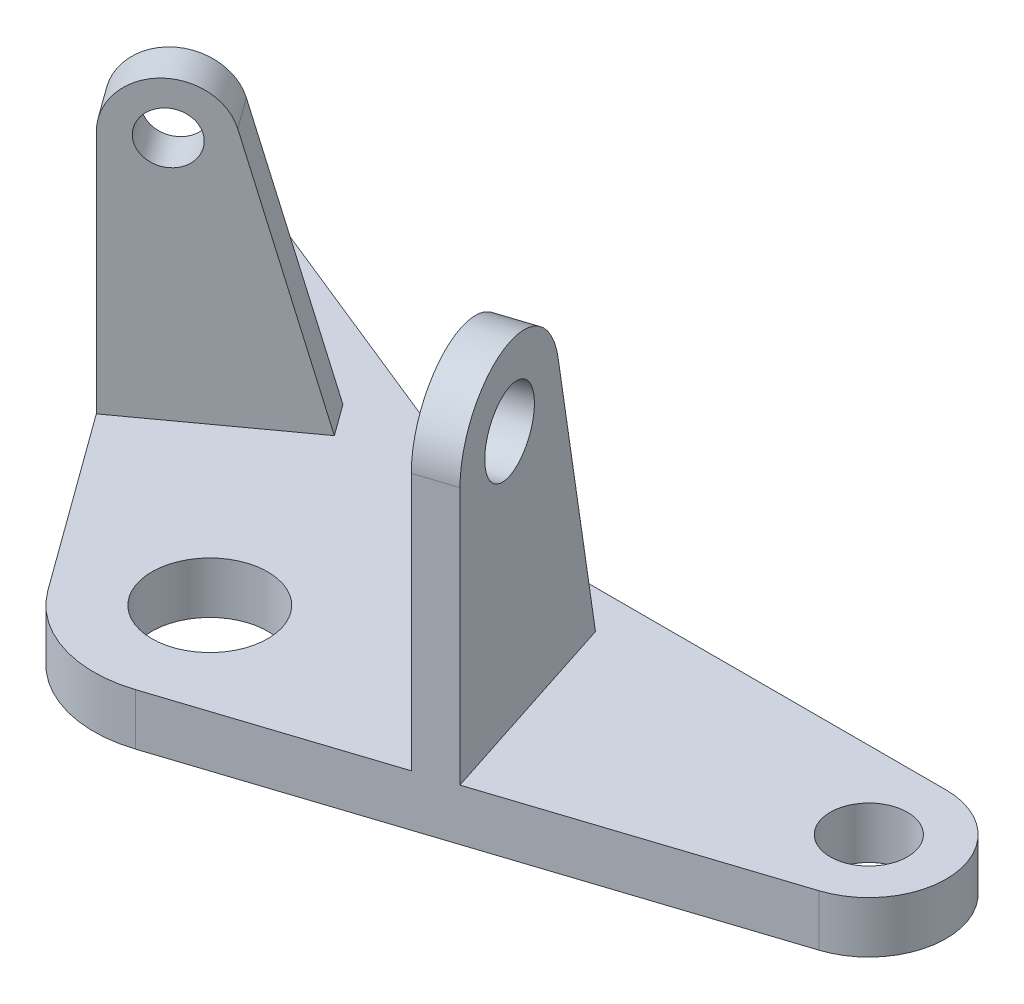
ISO-10303-21;
HEADER;
FILE_DESCRIPTION(('STEP AP214'),'2;1');
FILE_NAME('part.step','',(''),(''),'','','');
FILE_SCHEMA(('AUTOMOTIVE_DESIGN { 1 0 10303 214 1 1 1 1 }'));
ENDSEC;
DATA;
#1=APPLICATION_CONTEXT('core data for automotive mechanical design processes');
#2=APPLICATION_PROTOCOL_DEFINITION('international standard','automotive_design',2000,#1);
#3=PRODUCT_CONTEXT('',#1,'mechanical');
#4=PRODUCT('Part','Part','',(#3));
#5=PRODUCT_RELATED_PRODUCT_CATEGORY('part','',(#4));
#6=PRODUCT_DEFINITION_FORMATION('','',#4);
#7=PRODUCT_DEFINITION_CONTEXT('part definition',#1,'design');
#8=PRODUCT_DEFINITION('design','',#6,#7);
#9=PRODUCT_DEFINITION_SHAPE('','',#8);
#10=(LENGTH_UNIT() NAMED_UNIT(*) SI_UNIT(.MILLI.,.METRE.));
#11=(NAMED_UNIT(*) PLANE_ANGLE_UNIT() SI_UNIT($,.RADIAN.));
#12=(NAMED_UNIT(*) SI_UNIT($,.STERADIAN.) SOLID_ANGLE_UNIT());
#13=UNCERTAINTY_MEASURE_WITH_UNIT(LENGTH_MEASURE(1.E-05),#10,'distance_accuracy_value','');
#14=(GEOMETRIC_REPRESENTATION_CONTEXT(3) GLOBAL_UNCERTAINTY_ASSIGNED_CONTEXT((#13)) GLOBAL_UNIT_ASSIGNED_CONTEXT((#10,
#11,#12)) REPRESENTATION_CONTEXT('',''));
#15=CARTESIAN_POINT('',(0.,0.,0.));
#16=DIRECTION('',(0.,0.,1.));
#17=DIRECTION('',(1.,0.,0.));
#18=AXIS2_PLACEMENT_3D('',#15,#16,#17);
#19=CARTESIAN_POINT('',(82.,8.,-20.3346417456688));
#20=DIRECTION('',(0.,1.,0.));
#21=DIRECTION('',(0.,0.,1.));
#22=AXIS2_PLACEMENT_3D('',#19,#20,#21);
#23=PLANE('',#22);
#24=CARTESIAN_POINT('',(0.,8.,0.));
#25=DIRECTION('',(0.,1.,0.));
#26=DIRECTION('',(0.,0.,1.));
#27=AXIS2_PLACEMENT_3D('',#24,#25,#26);
#28=CIRCLE('',#27,9.);
#29=CARTESIAN_POINT('',(0.,8.,9.));
#30=VERTEX_POINT('',#29);
#31=EDGE_CURVE('E231',#30,#30,#28,.T.);
#32=ORIENTED_EDGE('',*,*,#31,.F.);
#33=EDGE_LOOP('',(#32));
#34=FACE_BOUND('',#33,.T.);
#35=CARTESIAN_POINT('',(82.,8.,-20.3346417456688));
#36=DIRECTION('',(0.,1.,0.));
#37=DIRECTION('',(0.,0.,1.));
#38=AXIS2_PLACEMENT_3D('',#35,#36,#37);
#39=CIRCLE('',#38,6.);
#40=CARTESIAN_POINT('',(82.,8.,-14.3346417456688));
#41=VERTEX_POINT('',#40);
#42=EDGE_CURVE('E227',#41,#41,#39,.T.);
#43=ORIENTED_EDGE('',*,*,#42,.F.);
#44=EDGE_LOOP('',(#43));
#45=FACE_BOUND('',#44,.T.);
#46=CARTESIAN_POINT('',(-48.,8.,-49.0533160155749));
#47=DIRECTION('',(0.,1.,0.));
#48=DIRECTION('',(0.,0.,1.));
#49=AXIS2_PLACEMENT_3D('',#46,#47,#48);
#50=CIRCLE('',#49,4.00000000000001);
#51=CARTESIAN_POINT('',(-48.,8.,-45.0533160155749));
#52=VERTEX_POINT('',#51);
#53=EDGE_CURVE('E223',#52,#52,#50,.T.);
#54=ORIENTED_EDGE('',*,*,#53,.F.);
#55=EDGE_LOOP('',(#54));
#56=FACE_BOUND('',#55,.T.);
#57=DIRECTION('',(0.309016994374949,0.,0.951056516295153));
#58=VECTOR('',#57,1.);
#59=CARTESIAN_POINT('',(37.8982274527843,8.,6.6124394845645));
#60=LINE('',#59,#58);
#61=CARTESIAN_POINT('',(27.7716325131749,8.,-24.5540150487136));
#62=VERTEX_POINT('',#61);
#63=CARTESIAN_POINT('',(37.8982274527843,8.,6.6124394845645));
#64=VERTEX_POINT('',#63);
#65=EDGE_CURVE('E54',#62,#64,#60,.T.);
#66=ORIENTED_EDGE('',*,*,#65,.F.);
#67=DIRECTION('',(0.951056516295153,0.,-0.309016994374949));
#68=VECTOR('',#67,1.);
#69=CARTESIAN_POINT('',(27.7716325131749,8.,-24.5540150487136));
#70=LINE('',#69,#68);
#71=CARTESIAN_POINT('',(33.4779716109458,8.,-26.4081170149633));
#72=VERTEX_POINT('',#71);
#73=EDGE_CURVE('E180',#62,#72,#70,.T.);
#74=ORIENTED_EDGE('',*,*,#73,.T.);
#75=DIRECTION('',(-0.309016994374949,0.,-0.951056516295153));
#76=VECTOR('',#75,1.);
#77=CARTESIAN_POINT('',(34.1624443371439,8.,-24.3015265738979));
#78=LINE('',#77,#76);
#79=CARTESIAN_POINT('',(43.6045665505552,8.,4.75833751831482));
#80=VERTEX_POINT('',#79);
#81=EDGE_CURVE('E64',#80,#72,#78,.T.);
#82=ORIENTED_EDGE('',*,*,#81,.F.);
#83=DIRECTION('',(0.951056516295153,0.,-0.309016994374949));
#84=VECTOR('',#83,1.);
#85=CARTESIAN_POINT('',(85.7082039324994,8.,-8.92196355012698));
#86=LINE('',#85,#84);
#87=CARTESIAN_POINT('',(85.7082039324994,8.,-8.92196355012698));
#88=VERTEX_POINT('',#87);
#89=EDGE_CURVE('E260',#80,#88,#86,.T.);
#90=ORIENTED_EDGE('',*,*,#89,.T.);
#91=CARTESIAN_POINT('',(82.,8.,-20.3346417456688));
#92=DIRECTION('',(0.,1.,0.));
#93=DIRECTION('',(0.,0.,1.));
#94=AXIS2_PLACEMENT_3D('',#91,#92,#93);
#95=CIRCLE('',#94,12.);
#96=CARTESIAN_POINT('',(82.,8.,-32.3346417456688));
#97=VERTEX_POINT('',#96);
#98=EDGE_CURVE('E237',#88,#97,#95,.T.);
#99=ORIENTED_EDGE('',*,*,#98,.T.);
#100=DIRECTION('',(-1.,0.,0.));
#101=VECTOR('',#100,1.);
#102=CARTESIAN_POINT('',(82.,8.,-32.3346417456688));
#103=LINE('',#102,#101);
#104=CARTESIAN_POINT('',(22.8998811762112,8.,-32.3346417456688));
#105=VERTEX_POINT('',#104);
#106=EDGE_CURVE('E245',#97,#105,#103,.T.);
#107=ORIENTED_EDGE('',*,*,#106,.T.);
#108=CARTESIAN_POINT('',(22.899881176211,8.,-74.3346417456688));
#109=DIRECTION('',(0.,-1.,0.));
#110=DIRECTION('',(0.,0.,-1.));
#111=AXIS2_PLACEMENT_3D('',#108,#109,#110);
#112=CIRCLE('',#111,42.);
#113=CARTESIAN_POINT('',(7.16640425274284,8.,-35.3929198538637));
#114=VERTEX_POINT('',#113);
#115=EDGE_CURVE('E244',#105,#114,#112,.T.);
#116=ORIENTED_EDGE('',*,*,#115,.T.);
#117=DIRECTION('',(-0.92718385456679,0.,-0.374606593415906));
#118=VECTOR('',#117,1.);
#119=CARTESIAN_POINT('',(-45.0031472526728,8.,-56.4707868521092));
#120=LINE('',#119,#118);
#121=CARTESIAN_POINT('',(-45.0031472526728,8.,-56.4707868521092));
#122=VERTEX_POINT('',#121);
#123=EDGE_CURVE('E250',#114,#122,#120,.T.);
#124=ORIENTED_EDGE('',*,*,#123,.T.);
#125=CARTESIAN_POINT('',(-48.,8.,-49.0533160155749));
#126=DIRECTION('',(0.,1.,0.));
#127=DIRECTION('',(0.,0.,1.));
#128=AXIS2_PLACEMENT_3D('',#125,#126,#127);
#129=CIRCLE('',#128,8.);
#130=CARTESIAN_POINT('',(-54.4721359549996,8.,-44.3510339972351));
#131=VERTEX_POINT('',#130);
#132=EDGE_CURVE('E248',#122,#131,#129,.T.);
#133=ORIENTED_EDGE('',*,*,#132,.T.);
#134=DIRECTION('',(0.587785252292478,0.,0.809016994374944));
#135=VECTOR('',#134,1.);
#136=CARTESIAN_POINT('',(-54.4721359549996,8.,-44.3510339972351));
#137=LINE('',#136,#135);
#138=CARTESIAN_POINT('',(-38.0737159904481,8.,-21.7805452337331));
#139=VERTEX_POINT('',#138);
#140=EDGE_CURVE('E255',#131,#139,#137,.T.);
#141=ORIENTED_EDGE('',*,*,#140,.T.);
#142=DIRECTION('',(-0.809016994374942,0.,0.58778525229248));
#143=VECTOR('',#142,1.);
#144=CARTESIAN_POINT('',(-14.333683815428,8.,-39.0286882251011));
#145=LINE('',#144,#143);
#146=CARTESIAN_POINT('',(-16.6636647332408,8.,-37.3358579988691));
#147=VERTEX_POINT('',#146);
#148=EDGE_CURVE('E206',#147,#139,#145,.T.);
#149=ORIENTED_EDGE('',*,*,#148,.F.);
#150=DIRECTION('',(-0.58778525229248,0.,-0.809016994374942));
#151=VECTOR('',#150,1.);
#152=CARTESIAN_POINT('',(40.9392899914223,8.,41.9478074498752));
#153=LINE('',#152,#151);
#154=CARTESIAN_POINT('',(-13.1369532194859,8.,-32.4817560326195));
#155=VERTEX_POINT('',#154);
#156=EDGE_CURVE('E189',#155,#147,#153,.T.);
#157=ORIENTED_EDGE('',*,*,#156,.F.);
#158=DIRECTION('',(0.809016994374942,0.,-0.58778525229248));
#159=VECTOR('',#158,1.);
#160=CARTESIAN_POINT('',(-34.5470044766932,8.,-16.9264432674835));
#161=LINE('',#160,#159);
#162=CARTESIAN_POINT('',(-34.5470044766932,8.,-16.9264432674835));
#163=VERTEX_POINT('',#162);
#164=EDGE_CURVE('E202',#163,#155,#161,.T.);
#165=ORIENTED_EDGE('',*,*,#164,.F.);
#166=CARTESIAN_POINT('',(-14.562305898749,8.,10.5801345412646));
#167=VERTEX_POINT('',#166);
#168=EDGE_CURVE('E252',#163,#167,#137,.T.);
#169=ORIENTED_EDGE('',*,*,#168,.T.);
#170=CARTESIAN_POINT('',(0.,8.,0.));
#171=DIRECTION('',(0.,1.,0.));
#172=DIRECTION('',(0.,0.,1.));
#173=AXIS2_PLACEMENT_3D('',#170,#171,#172);
#174=CIRCLE('',#173,18.);
#175=CARTESIAN_POINT('',(5.56230589874908,8.,17.1190172933128));
#176=VERTEX_POINT('',#175);
#177=EDGE_CURVE('E253',#167,#176,#174,.T.);
#178=ORIENTED_EDGE('',*,*,#177,.T.);
#179=EDGE_CURVE('E259',#176,#64,#86,.T.);
#180=ORIENTED_EDGE('',*,*,#179,.T.);
#181=EDGE_LOOP('',(#66,#74,#82,#90,#99,#107,#116,#124,#133,#141,#149,#157,#165,#169,#178,#180));
#182=FACE_BOUND('',#181,.T.);
#183=ADVANCED_FACE('F39',(#34,#45,#56,#182),#23,.T.);
#184=CARTESIAN_POINT('',(-54.4721359549996,8.,-44.3510339972351));
#185=DIRECTION('',(0.809016994374944,0.,-0.587785252292478));
#186=DIRECTION('',(-0.587785252292478,0.,-0.809016994374944));
#187=AXIS2_PLACEMENT_3D('',#184,#185,#186);
#188=PLANE('',#187);
#189=DIRECTION('',(-0.58778525229248,0.,-0.809016994374942));
#190=VECTOR('',#189,1.);
#191=CARTESIAN_POINT('',(19.529238734215,46.,57.5031202150112));
#192=LINE('',#191,#190);
#193=CARTESIAN_POINT('',(-34.5470044766932,46.,-16.9264432674835));
#194=VERTEX_POINT('',#193);
#195=CARTESIAN_POINT('',(-38.0737159904481,46.,-21.7805452337331));
#196=VERTEX_POINT('',#195);
#197=EDGE_CURVE('E186',#194,#196,#192,.T.);
#198=ORIENTED_EDGE('',*,*,#197,.T.);
#199=DIRECTION('',(0.,-1.,0.));
#200=VECTOR('',#199,1.);
#201=CARTESIAN_POINT('',(-38.0737159904481,106.,-21.7805452337331));
#202=LINE('',#201,#200);
#203=EDGE_CURVE('E212',#196,#139,#202,.T.);
#204=ORIENTED_EDGE('',*,*,#203,.T.);
#205=ORIENTED_EDGE('',*,*,#140,.F.);
#206=DIRECTION('',(0.,-1.,0.));
#207=VECTOR('',#206,1.);
#208=CARTESIAN_POINT('',(-54.4721359549996,8.,-44.3510339972351));
#209=LINE('',#208,#207);
#210=CARTESIAN_POINT('',(-54.4721359549996,0.,-44.3510339972351));
#211=VERTEX_POINT('',#210);
#212=EDGE_CURVE('E283',#131,#211,#209,.T.);
#213=ORIENTED_EDGE('',*,*,#212,.T.);
#214=DIRECTION('',(0.587785252292478,0.,0.809016994374944));
#215=VECTOR('',#214,1.);
#216=CARTESIAN_POINT('',(-54.4721359549996,0.,-44.3510339972351));
#217=LINE('',#216,#215);
#218=CARTESIAN_POINT('',(-14.562305898749,0.,10.5801345412646));
#219=VERTEX_POINT('',#218);
#220=EDGE_CURVE('E272',#211,#219,#217,.T.);
#221=ORIENTED_EDGE('',*,*,#220,.T.);
#222=DIRECTION('',(0.,-1.,0.));
#223=VECTOR('',#222,1.);
#224=CARTESIAN_POINT('',(-14.562305898749,8.,10.5801345412646));
#225=LINE('',#224,#223);
#226=EDGE_CURVE('E284',#167,#219,#225,.T.);
#227=ORIENTED_EDGE('',*,*,#226,.F.);
#228=ORIENTED_EDGE('',*,*,#168,.F.);
#229=DIRECTION('',(0.,-1.,0.));
#230=VECTOR('',#229,1.);
#231=CARTESIAN_POINT('',(-34.5470044766932,106.,-16.9264432674835));
#232=LINE('',#231,#230);
#233=EDGE_CURVE('E214',#194,#163,#232,.T.);
#234=ORIENTED_EDGE('',*,*,#233,.F.);
#235=EDGE_LOOP('',(#198,#204,#205,#213,#221,#227,#228,#234));
#236=FACE_BOUND('',#235,.T.);
#237=ADVANCED_FACE('F334',(#236),#188,.F.);
#238=CARTESIAN_POINT('',(82.,0.,-20.3346417456688));
#239=DIRECTION('',(0.,1.,0.));
#240=DIRECTION('',(0.,0.,1.));
#241=AXIS2_PLACEMENT_3D('',#238,#239,#240);
#242=PLANE('',#241);
#243=CARTESIAN_POINT('',(82.,0.,-20.3346417456688));
#244=DIRECTION('',(0.,1.,0.));
#245=DIRECTION('',(0.,0.,1.));
#246=AXIS2_PLACEMENT_3D('',#243,#244,#245);
#247=CIRCLE('',#246,12.);
#248=CARTESIAN_POINT('',(85.7082039324994,0.,-8.92196355012698));
#249=VERTEX_POINT('',#248);
#250=CARTESIAN_POINT('',(82.,0.,-32.3346417456688));
#251=VERTEX_POINT('',#250);
#252=EDGE_CURVE('E236',#249,#251,#247,.T.);
#253=ORIENTED_EDGE('',*,*,#252,.F.);
#254=DIRECTION('',(0.951056516295153,0.,-0.309016994374949));
#255=VECTOR('',#254,1.);
#256=CARTESIAN_POINT('',(85.7082039324994,0.,-8.92196355012698));
#257=LINE('',#256,#255);
#258=CARTESIAN_POINT('',(5.56230589874908,0.,17.1190172933128));
#259=VERTEX_POINT('',#258);
#260=EDGE_CURVE('E243',#259,#249,#257,.T.);
#261=ORIENTED_EDGE('',*,*,#260,.F.);
#262=CARTESIAN_POINT('',(0.,0.,0.));
#263=DIRECTION('',(0.,1.,0.));
#264=DIRECTION('',(0.,0.,1.));
#265=AXIS2_PLACEMENT_3D('',#262,#263,#264);
#266=CIRCLE('',#265,18.);
#267=EDGE_CURVE('E271',#219,#259,#266,.T.);
#268=ORIENTED_EDGE('',*,*,#267,.F.);
#269=ORIENTED_EDGE('',*,*,#220,.F.);
#270=CARTESIAN_POINT('',(-48.,0.,-49.0533160155749));
#271=DIRECTION('',(0.,1.,0.));
#272=DIRECTION('',(0.,0.,1.));
#273=AXIS2_PLACEMENT_3D('',#270,#271,#272);
#274=CIRCLE('',#273,8.);
#275=CARTESIAN_POINT('',(-45.0031472526728,0.,-56.4707868521092));
#276=VERTEX_POINT('',#275);
#277=EDGE_CURVE('E269',#276,#211,#274,.T.);
#278=ORIENTED_EDGE('',*,*,#277,.F.);
#279=DIRECTION('',(-0.92718385456679,0.,-0.374606593415906));
#280=VECTOR('',#279,1.);
#281=CARTESIAN_POINT('',(-45.0031472526728,0.,-56.4707868521092));
#282=LINE('',#281,#280);
#283=CARTESIAN_POINT('',(7.16640425274284,0.,-35.3929198538637));
#284=VERTEX_POINT('',#283);
#285=EDGE_CURVE('E270',#284,#276,#282,.T.);
#286=ORIENTED_EDGE('',*,*,#285,.F.);
#287=CARTESIAN_POINT('',(22.899881176211,0.,-74.3346417456688));
#288=DIRECTION('',(0.,-1.,0.));
#289=DIRECTION('',(0.,0.,-1.));
#290=AXIS2_PLACEMENT_3D('',#287,#288,#289);
#291=CIRCLE('',#290,42.);
#292=CARTESIAN_POINT('',(22.8998811762112,0.,-32.3346417456688));
#293=VERTEX_POINT('',#292);
#294=EDGE_CURVE('E262',#293,#284,#291,.T.);
#295=ORIENTED_EDGE('',*,*,#294,.F.);
#296=DIRECTION('',(-1.,0.,0.));
#297=VECTOR('',#296,1.);
#298=CARTESIAN_POINT('',(82.,0.,-32.3346417456688));
#299=LINE('',#298,#297);
#300=EDGE_CURVE('E265',#251,#293,#299,.T.);
#301=ORIENTED_EDGE('',*,*,#300,.F.);
#302=EDGE_LOOP('',(#253,#261,#268,#269,#278,#286,#295,#301));
#303=FACE_BOUND('',#302,.T.);
#304=CARTESIAN_POINT('',(0.,0.,0.));
#305=DIRECTION('',(0.,1.,0.));
#306=DIRECTION('',(0.,0.,1.));
#307=AXIS2_PLACEMENT_3D('',#304,#305,#306);
#308=CIRCLE('',#307,9.);
#309=CARTESIAN_POINT('',(0.,0.,9.));
#310=VERTEX_POINT('',#309);
#311=EDGE_CURVE('E229',#310,#310,#308,.T.);
#312=ORIENTED_EDGE('',*,*,#311,.T.);
#313=EDGE_LOOP('',(#312));
#314=FACE_BOUND('',#313,.T.);
#315=CARTESIAN_POINT('',(82.,0.,-20.3346417456688));
#316=DIRECTION('',(0.,1.,0.));
#317=DIRECTION('',(0.,0.,1.));
#318=AXIS2_PLACEMENT_3D('',#315,#316,#317);
#319=CIRCLE('',#318,6.);
#320=CARTESIAN_POINT('',(82.,0.,-14.3346417456688));
#321=VERTEX_POINT('',#320);
#322=EDGE_CURVE('E224',#321,#321,#319,.T.);
#323=ORIENTED_EDGE('',*,*,#322,.T.);
#324=EDGE_LOOP('',(#323));
#325=FACE_BOUND('',#324,.T.);
#326=CARTESIAN_POINT('',(-48.,0.,-49.0533160155749));
#327=DIRECTION('',(0.,1.,0.));
#328=DIRECTION('',(0.,0.,1.));
#329=AXIS2_PLACEMENT_3D('',#326,#327,#328);
#330=CIRCLE('',#329,4.00000000000001);
#331=CARTESIAN_POINT('',(-48.,0.,-45.0533160155749));
#332=VERTEX_POINT('',#331);
#333=EDGE_CURVE('E213',#332,#332,#330,.T.);
#334=ORIENTED_EDGE('',*,*,#333,.T.);
#335=EDGE_LOOP('',(#334));
#336=FACE_BOUND('',#335,.T.);
#337=ADVANCED_FACE('F310',(#303,#314,#325,#336),#242,.F.);
#338=CARTESIAN_POINT('',(82.,8.,-20.3346417456688));
#339=DIRECTION('',(0.,-1.,0.));
#340=DIRECTION('',(0.,0.,-1.));
#341=AXIS2_PLACEMENT_3D('',#338,#339,#340);
#342=CYLINDRICAL_SURFACE('',#341,12.);
#343=ORIENTED_EDGE('',*,*,#252,.T.);
#344=DIRECTION('',(0.,-1.,0.));
#345=VECTOR('',#344,1.);
#346=CARTESIAN_POINT('',(82.,8.,-32.3346417456688));
#347=LINE('',#346,#345);
#348=EDGE_CURVE('E48',#97,#251,#347,.T.);
#349=ORIENTED_EDGE('',*,*,#348,.F.);
#350=ORIENTED_EDGE('',*,*,#98,.F.);
#351=DIRECTION('',(0.,-1.,0.));
#352=VECTOR('',#351,1.);
#353=CARTESIAN_POINT('',(85.7082039324994,8.,-8.92196355012698));
#354=LINE('',#353,#352);
#355=EDGE_CURVE('E258',#88,#249,#354,.T.);
#356=ORIENTED_EDGE('',*,*,#355,.T.);
#357=EDGE_LOOP('',(#343,#349,#350,#356));
#358=FACE_BOUND('',#357,.T.);
#359=ADVANCED_FACE('F41',(#358),#342,.T.);
#360=CARTESIAN_POINT('',(82.,8.,-32.3346417456688));
#361=DIRECTION('',(0.,0.,1.));
#362=DIRECTION('',(1.,0.,0.));
#363=AXIS2_PLACEMENT_3D('',#360,#361,#362);
#364=PLANE('',#363);
#365=ORIENTED_EDGE('',*,*,#300,.T.);
#366=DIRECTION('',(0.,-1.,0.));
#367=VECTOR('',#366,1.);
#368=CARTESIAN_POINT('',(22.8998811762112,8.,-32.3346417456688));
#369=LINE('',#368,#367);
#370=EDGE_CURVE('E291',#105,#293,#369,.T.);
#371=ORIENTED_EDGE('',*,*,#370,.F.);
#372=ORIENTED_EDGE('',*,*,#106,.F.);
#373=ORIENTED_EDGE('',*,*,#348,.T.);
#374=EDGE_LOOP('',(#365,#371,#372,#373));
#375=FACE_BOUND('',#374,.T.);
#376=ADVANCED_FACE('F299',(#375),#364,.F.);
#377=CARTESIAN_POINT('',(22.899881176211,8.,-74.3346417456688));
#378=DIRECTION('',(0.,-1.,0.));
#379=DIRECTION('',(0.,0.,-1.));
#380=AXIS2_PLACEMENT_3D('',#377,#378,#379);
#381=CYLINDRICAL_SURFACE('',#380,42.);
#382=ORIENTED_EDGE('',*,*,#294,.T.);
#383=DIRECTION('',(0.,-1.,0.));
#384=VECTOR('',#383,1.);
#385=CARTESIAN_POINT('',(7.16640425274284,8.,-35.3929198538637));
#386=LINE('',#385,#384);
#387=EDGE_CURVE('E287',#114,#284,#386,.T.);
#388=ORIENTED_EDGE('',*,*,#387,.F.);
#389=ORIENTED_EDGE('',*,*,#115,.F.);
#390=ORIENTED_EDGE('',*,*,#370,.T.);
#391=EDGE_LOOP('',(#382,#388,#389,#390));
#392=FACE_BOUND('',#391,.T.);
#393=ADVANCED_FACE('F314',(#392),#381,.F.);
#394=CARTESIAN_POINT('',(-45.0031472526728,8.,-56.4707868521092));
#395=DIRECTION('',(-0.374606593415906,0.,0.92718385456679));
#396=DIRECTION('',(0.92718385456679,0.,0.374606593415906));
#397=AXIS2_PLACEMENT_3D('',#394,#395,#396);
#398=PLANE('',#397);
#399=ORIENTED_EDGE('',*,*,#285,.T.);
#400=DIRECTION('',(0.,-1.,0.));
#401=VECTOR('',#400,1.);
#402=CARTESIAN_POINT('',(-45.0031472526728,8.,-56.4707868521092));
#403=LINE('',#402,#401);
#404=EDGE_CURVE('E290',#122,#276,#403,.T.);
#405=ORIENTED_EDGE('',*,*,#404,.F.);
#406=ORIENTED_EDGE('',*,*,#123,.F.);
#407=ORIENTED_EDGE('',*,*,#387,.T.);
#408=EDGE_LOOP('',(#399,#405,#406,#407));
#409=FACE_BOUND('',#408,.T.);
#410=ADVANCED_FACE('F316',(#409),#398,.F.);
#411=CARTESIAN_POINT('',(-48.,8.,-49.0533160155749));
#412=DIRECTION('',(0.,-1.,0.));
#413=DIRECTION('',(0.,0.,-1.));
#414=AXIS2_PLACEMENT_3D('',#411,#412,#413);
#415=CYLINDRICAL_SURFACE('',#414,8.);
#416=ORIENTED_EDGE('',*,*,#277,.T.);
#417=ORIENTED_EDGE('',*,*,#212,.F.);
#418=ORIENTED_EDGE('',*,*,#132,.F.);
#419=ORIENTED_EDGE('',*,*,#404,.T.);
#420=EDGE_LOOP('',(#416,#417,#418,#419));
#421=FACE_BOUND('',#420,.T.);
#422=ADVANCED_FACE('F336',(#421),#415,.T.);
#423=CARTESIAN_POINT('',(0.,8.,0.));
#424=DIRECTION('',(0.,-1.,0.));
#425=DIRECTION('',(0.,0.,-1.));
#426=AXIS2_PLACEMENT_3D('',#423,#424,#425);
#427=CYLINDRICAL_SURFACE('',#426,18.);
#428=ORIENTED_EDGE('',*,*,#267,.T.);
#429=DIRECTION('',(0.,-1.,0.));
#430=VECTOR('',#429,1.);
#431=CARTESIAN_POINT('',(5.56230589874908,8.,17.1190172933128));
#432=LINE('',#431,#430);
#433=EDGE_CURVE('E279',#176,#259,#432,.T.);
#434=ORIENTED_EDGE('',*,*,#433,.F.);
#435=ORIENTED_EDGE('',*,*,#177,.F.);
#436=ORIENTED_EDGE('',*,*,#226,.T.);
#437=EDGE_LOOP('',(#428,#434,#435,#436));
#438=FACE_BOUND('',#437,.T.);
#439=ADVANCED_FACE('F327',(#438),#427,.T.);
#440=CARTESIAN_POINT('',(85.7082039324994,8.,-8.92196355012698));
#441=DIRECTION('',(-0.309016994374949,0.,-0.951056516295153));
#442=DIRECTION('',(-0.951056516295153,0.,0.309016994374949));
#443=AXIS2_PLACEMENT_3D('',#440,#441,#442);
#444=PLANE('',#443);
#445=DIRECTION('',(0.,-1.,0.));
#446=VECTOR('',#445,1.);
#447=CARTESIAN_POINT('',(43.6045665505552,106.,4.75833751831481));
#448=LINE('',#447,#446);
#449=CARTESIAN_POINT('',(43.6045665505552,48.,4.75833751831482));
#450=VERTEX_POINT('',#449);
#451=EDGE_CURVE('E204',#450,#80,#448,.T.);
#452=ORIENTED_EDGE('',*,*,#451,.F.);
#453=DIRECTION('',(0.951056516295153,0.,-0.309016994374949));
#454=VECTOR('',#453,1.);
#455=CARTESIAN_POINT('',(28.3876622898328,48.,9.702609428314));
#456=LINE('',#455,#454);
#457=CARTESIAN_POINT('',(37.8982274527843,48.,6.61243948456451));
#458=VERTEX_POINT('',#457);
#459=EDGE_CURVE('E170',#458,#450,#456,.T.);
#460=ORIENTED_EDGE('',*,*,#459,.F.);
#461=DIRECTION('',(0.,-1.,0.));
#462=VECTOR('',#461,1.);
#463=CARTESIAN_POINT('',(37.8982274527843,106.,6.6124394845645));
#464=LINE('',#463,#462);
#465=EDGE_CURVE('E216',#458,#64,#464,.T.);
#466=ORIENTED_EDGE('',*,*,#465,.T.);
#467=ORIENTED_EDGE('',*,*,#179,.F.);
#468=ORIENTED_EDGE('',*,*,#433,.T.);
#469=ORIENTED_EDGE('',*,*,#260,.T.);
#470=ORIENTED_EDGE('',*,*,#355,.F.);
#471=ORIENTED_EDGE('',*,*,#89,.F.);
#472=EDGE_LOOP('',(#452,#460,#466,#467,#468,#469,#470,#471));
#473=FACE_BOUND('',#472,.T.);
#474=ADVANCED_FACE('F323',(#473),#444,.F.);
#475=CARTESIAN_POINT('',(0.,8.,0.));
#476=DIRECTION('',(0.,-1.,0.));
#477=DIRECTION('',(0.,0.,-1.));
#478=AXIS2_PLACEMENT_3D('',#475,#476,#477);
#479=CYLINDRICAL_SURFACE('',#478,9.);
#480=ORIENTED_EDGE('',*,*,#31,.T.);
#481=EDGE_LOOP('',(#480));
#482=FACE_BOUND('',#481,.T.);
#483=ORIENTED_EDGE('',*,*,#311,.F.);
#484=EDGE_LOOP('',(#483));
#485=FACE_BOUND('',#484,.T.);
#486=ADVANCED_FACE('F359',(#482,#485),#479,.F.);
#487=CARTESIAN_POINT('',(82.,8.,-20.3346417456688));
#488=DIRECTION('',(0.,-1.,0.));
#489=DIRECTION('',(0.,0.,-1.));
#490=AXIS2_PLACEMENT_3D('',#487,#488,#489);
#491=CYLINDRICAL_SURFACE('',#490,6.);
#492=ORIENTED_EDGE('',*,*,#42,.T.);
#493=EDGE_LOOP('',(#492));
#494=FACE_BOUND('',#493,.T.);
#495=ORIENTED_EDGE('',*,*,#322,.F.);
#496=EDGE_LOOP('',(#495));
#497=FACE_BOUND('',#496,.T.);
#498=ADVANCED_FACE('F368',(#494,#497),#491,.F.);
#499=CARTESIAN_POINT('',(-48.,8.,-49.0533160155749));
#500=DIRECTION('',(0.,-1.,0.));
#501=DIRECTION('',(0.,0.,-1.));
#502=AXIS2_PLACEMENT_3D('',#499,#500,#501);
#503=CYLINDRICAL_SURFACE('',#502,4.00000000000001);
#504=ORIENTED_EDGE('',*,*,#53,.T.);
#505=EDGE_LOOP('',(#504));
#506=FACE_BOUND('',#505,.T.);
#507=ORIENTED_EDGE('',*,*,#333,.F.);
#508=EDGE_LOOP('',(#507));
#509=FACE_BOUND('',#508,.T.);
#510=ADVANCED_FACE('F372',(#506,#509),#503,.F.);
#511=CARTESIAN_POINT('',(34.1624443371439,106.,-24.3015265738979));
#512=DIRECTION('',(-0.951056516295153,0.,0.309016994374949));
#513=DIRECTION('',(0.309016994374949,0.,0.951056516295153));
#514=AXIS2_PLACEMENT_3D('',#511,#512,#513);
#515=PLANE('',#514);
#516=CARTESIAN_POINT('',(39.8963626180558,48.,-6.65434067722702));
#517=DIRECTION('',(0.951056516295153,0.,-0.309016994374949));
#518=DIRECTION('',(-0.309016994374949,0.,-0.951056516295153));
#519=AXIS2_PLACEMENT_3D('',#516,#517,#518);
#520=CIRCLE('',#519,6.);
#521=CARTESIAN_POINT('',(38.0422606518062,48.,-12.3606797749979));
#522=VERTEX_POINT('',#521);
#523=EDGE_CURVE('E171',#522,#522,#520,.T.);
#524=ORIENTED_EDGE('',*,*,#523,.F.);
#525=EDGE_LOOP('',(#524));
#526=FACE_BOUND('',#525,.T.);
#527=DIRECTION('',(0.0642482457919188,0.978147600733805,0.197735768366177));
#528=VECTOR('',#527,1.);
#529=CARTESIAN_POINT('',(33.4779716109458,8.,-26.4081170149633));
#530=LINE('',#529,#528);
#531=CARTESIAN_POINT('',(36.2691918384499,50.4949402898132,-17.8176244721433));
#532=VERTEX_POINT('',#531);
#533=EDGE_CURVE('E155',#72,#532,#530,.T.);
#534=ORIENTED_EDGE('',*,*,#533,.T.);
#535=CARTESIAN_POINT('',(39.8963626180558,48.,-6.65434067722702));
#536=DIRECTION('',(-0.951056516295153,0.,0.309016994374949));
#537=DIRECTION('',(-0.309016994374949,0.,-0.951056516295153));
#538=AXIS2_PLACEMENT_3D('',#535,#536,#537);
#539=CIRCLE('',#538,12.);
#540=EDGE_CURVE('E160',#450,#532,#539,.T.);
#541=ORIENTED_EDGE('',*,*,#540,.F.);
#542=ORIENTED_EDGE('',*,*,#451,.T.);
#543=ORIENTED_EDGE('',*,*,#81,.T.);
#544=EDGE_LOOP('',(#534,#541,#542,#543));
#545=FACE_BOUND('',#544,.T.);
#546=ADVANCED_FACE('F152',(#526,#545),#515,.F.);
#547=CARTESIAN_POINT('',(37.8982274527843,106.,6.6124394845645));
#548=DIRECTION('',(0.951056516295153,0.,-0.309016994374949));
#549=DIRECTION('',(-0.30901699437495,0.,-0.951056516295153));
#550=AXIS2_PLACEMENT_3D('',#547,#548,#549);
#551=PLANE('',#550);
#552=CARTESIAN_POINT('',(34.1900235202849,48.,-4.80023871097732));
#553=DIRECTION('',(0.951056516295153,0.,-0.309016994374949));
#554=DIRECTION('',(-0.30901699437495,0.,-0.951056516295153));
#555=AXIS2_PLACEMENT_3D('',#552,#553,#554);
#556=CIRCLE('',#555,6.);
#557=CARTESIAN_POINT('',(32.3359215540352,48.,-10.5065778087482));
#558=VERTEX_POINT('',#557);
#559=EDGE_CURVE('E43',#558,#558,#556,.T.);
#560=ORIENTED_EDGE('',*,*,#559,.T.);
#561=EDGE_LOOP('',(#560));
#562=FACE_BOUND('',#561,.T.);
#563=ORIENTED_EDGE('',*,*,#465,.F.);
#564=CARTESIAN_POINT('',(34.1900235202849,48.,-4.80023871097732));
#565=DIRECTION('',(0.951056516295153,0.,-0.309016994374949));
#566=DIRECTION('',(-0.30901699437495,0.,-0.951056516295153));
#567=AXIS2_PLACEMENT_3D('',#564,#565,#566);
#568=CIRCLE('',#567,12.);
#569=CARTESIAN_POINT('',(30.562852740679,50.4949402898132,-15.9635225058936));
#570=VERTEX_POINT('',#569);
#571=EDGE_CURVE('E11',#458,#570,#568,.F.);
#572=ORIENTED_EDGE('',*,*,#571,.T.);
#573=DIRECTION('',(0.0642482457919188,0.978147600733805,0.197735768366177));
#574=VECTOR('',#573,1.);
#575=CARTESIAN_POINT('',(27.7716325131749,8.,-24.5540150487136));
#576=LINE('',#575,#574);
#577=EDGE_CURVE('E157',#62,#570,#576,.T.);
#578=ORIENTED_EDGE('',*,*,#577,.F.);
#579=ORIENTED_EDGE('',*,*,#65,.T.);
#580=EDGE_LOOP('',(#563,#572,#578,#579));
#581=FACE_BOUND('',#580,.T.);
#582=ADVANCED_FACE('F389',(#562,#581),#551,.F.);
#583=CARTESIAN_POINT('',(-34.5470044766932,106.,-16.9264432674835));
#584=DIRECTION('',(-0.58778525229248,0.,-0.809016994374942));
#585=DIRECTION('',(-0.809016994374942,0.,0.58778525229248));
#586=AXIS2_PLACEMENT_3D('',#583,#584,#585);
#587=PLANE('',#586);
#588=CARTESIAN_POINT('',(-28.0748685216936,46.,-21.6287252858233));
#589=DIRECTION('',(-0.58778525229248,0.,-0.809016994374942));
#590=DIRECTION('',(-0.809016994374942,0.,0.58778525229248));
#591=AXIS2_PLACEMENT_3D('',#588,#589,#590);
#592=CIRCLE('',#591,4.);
#593=CARTESIAN_POINT('',(-31.3109364991934,46.,-19.2775842766534));
#594=VERTEX_POINT('',#593);
#595=EDGE_CURVE('E203',#594,#594,#592,.T.);
#596=ORIENTED_EDGE('',*,*,#595,.T.);
#597=EDGE_LOOP('',(#596));
#598=FACE_BOUND('',#597,.T.);
#599=DIRECTION('',(-0.209389005955832,0.965925826289069,0.152130017723682));
#600=VECTOR('',#599,1.);
#601=CARTESIAN_POINT('',(-34.3920710677412,106.051314474353,-17.039008978096));
#602=LINE('',#601,#600);
#603=CARTESIAN_POINT('',(-21.8232652515055,48.0705523608201,-26.1707809298324));
#604=VERTEX_POINT('',#603);
#605=EDGE_CURVE('E195',#155,#604,#602,.T.);
#606=ORIENTED_EDGE('',*,*,#605,.T.);
#607=CARTESIAN_POINT('',(-28.0748685216936,46.,-21.6287252858233));
#608=DIRECTION('',(-0.58778525229248,0.,-0.809016994374942));
#609=DIRECTION('',(-0.809016994374942,0.,0.58778525229248));
#610=AXIS2_PLACEMENT_3D('',#607,#608,#609);
#611=CIRCLE('',#610,8.);
#612=EDGE_CURVE('E200',#604,#194,#611,.F.);
#613=ORIENTED_EDGE('',*,*,#612,.T.);
#614=ORIENTED_EDGE('',*,*,#233,.T.);
#615=ORIENTED_EDGE('',*,*,#164,.T.);
#616=EDGE_LOOP('',(#606,#613,#614,#615));
#617=FACE_BOUND('',#616,.T.);
#618=ADVANCED_FACE('F395',(#598,#617),#587,.F.);
#619=CARTESIAN_POINT('',(-14.333683815428,106.,-39.0286882251011));
#620=DIRECTION('',(0.587785252292481,0.,0.809016994374942));
#621=DIRECTION('',(0.809016994374942,0.,-0.58778525229248));
#622=AXIS2_PLACEMENT_3D('',#619,#620,#621);
#623=PLANE('',#622);
#624=CARTESIAN_POINT('',(-31.6015800354485,46.,-26.482827252073));
#625=DIRECTION('',(-0.58778525229248,0.,-0.809016994374942));
#626=DIRECTION('',(-0.809016994374942,0.,0.58778525229248));
#627=AXIS2_PLACEMENT_3D('',#624,#625,#626);
#628=CIRCLE('',#627,4.);
#629=CARTESIAN_POINT('',(-34.8376480129483,46.,-24.1316862429031));
#630=VERTEX_POINT('',#629);
#631=EDGE_CURVE('E179',#630,#630,#628,.T.);
#632=ORIENTED_EDGE('',*,*,#631,.F.);
#633=EDGE_LOOP('',(#632));
#634=FACE_BOUND('',#633,.T.);
#635=ORIENTED_EDGE('',*,*,#203,.F.);
#636=CARTESIAN_POINT('',(-31.6015800354485,46.,-26.482827252073));
#637=DIRECTION('',(0.58778525229248,0.,0.809016994374942));
#638=DIRECTION('',(-0.809016994374942,0.,0.58778525229248));
#639=AXIS2_PLACEMENT_3D('',#636,#637,#638);
#640=CIRCLE('',#639,8.);
#641=CARTESIAN_POINT('',(-25.3499767652604,48.0705523608201,-31.0248828960821));
#642=VERTEX_POINT('',#641);
#643=EDGE_CURVE('E187',#642,#196,#640,.T.);
#644=ORIENTED_EDGE('',*,*,#643,.F.);
#645=DIRECTION('',(-0.209389005955831,0.965925826289069,0.152130017723682));
#646=VECTOR('',#645,1.);
#647=CARTESIAN_POINT('',(-16.6636647332408,8.,-37.3358579988691));
#648=LINE('',#647,#646);
#649=EDGE_CURVE('E182',#147,#642,#648,.T.);
#650=ORIENTED_EDGE('',*,*,#649,.F.);
#651=ORIENTED_EDGE('',*,*,#148,.T.);
#652=EDGE_LOOP('',(#635,#644,#650,#651));
#653=FACE_BOUND('',#652,.T.);
#654=ADVANCED_FACE('F400',(#634,#653),#623,.F.);
#655=CARTESIAN_POINT('',(26.0013746892145,46.,52.8008381966714));
#656=DIRECTION('',(-0.58778525229248,0.,-0.809016994374942));
#657=DIRECTION('',(-0.809016994374942,0.,0.58778525229248));
#658=AXIS2_PLACEMENT_3D('',#655,#656,#657);
#659=CYLINDRICAL_SURFACE('',#658,8.);
#660=DIRECTION('',(-0.58778525229248,0.,-0.809016994374942));
#661=VECTOR('',#660,1.);
#662=CARTESIAN_POINT('',(32.2529779594027,48.0705523608201,48.2587825526622));
#663=LINE('',#662,#661);
#664=EDGE_CURVE('E194',#604,#642,#663,.T.);
#665=ORIENTED_EDGE('',*,*,#664,.T.);
#666=ORIENTED_EDGE('',*,*,#643,.T.);
#667=ORIENTED_EDGE('',*,*,#197,.F.);
#668=ORIENTED_EDGE('',*,*,#612,.F.);
#669=EDGE_LOOP('',(#665,#666,#667,#668));
#670=FACE_BOUND('',#669,.T.);
#671=ADVANCED_FACE('F402',(#670),#659,.T.);
#672=CARTESIAN_POINT('',(40.9392899914223,8.,41.9478074498752));
#673=DIRECTION('',(-0.781450408773515,-0.258819045102518,0.567756955501143));
#674=DIRECTION('',(0.58778525229248,0.,0.809016994374942));
#675=AXIS2_PLACEMENT_3D('',#672,#673,#674);
#676=PLANE('',#675);
#677=ORIENTED_EDGE('',*,*,#156,.T.);
#678=ORIENTED_EDGE('',*,*,#649,.T.);
#679=ORIENTED_EDGE('',*,*,#664,.F.);
#680=ORIENTED_EDGE('',*,*,#605,.F.);
#681=EDGE_LOOP('',(#677,#678,#679,#680));
#682=FACE_BOUND('',#681,.T.);
#683=ADVANCED_FACE('F401',(#682),#676,.F.);
#684=CARTESIAN_POINT('',(26.0013746892145,46.,52.8008381966714));
#685=DIRECTION('',(-0.58778525229248,0.,-0.809016994374942));
#686=DIRECTION('',(-0.809016994374942,0.,0.58778525229248));
#687=AXIS2_PLACEMENT_3D('',#684,#685,#686);
#688=CYLINDRICAL_SURFACE('',#687,4.);
#689=ORIENTED_EDGE('',*,*,#631,.T.);
#690=EDGE_LOOP('',(#689));
#691=FACE_BOUND('',#690,.T.);
#692=ORIENTED_EDGE('',*,*,#595,.F.);
#693=EDGE_LOOP('',(#692));
#694=FACE_BOUND('',#693,.T.);
#695=ADVANCED_FACE('F407',(#691,#694),#688,.F.);
#696=CARTESIAN_POINT('',(27.7716325131749,8.,-24.5540150487136));
#697=DIRECTION('',(-0.302264231633828,0.207911690817763,-0.930273649576355));
#698=DIRECTION('',(-0.951056516295153,0.,0.309016994374949));
#699=AXIS2_PLACEMENT_3D('',#696,#697,#698);
#700=PLANE('',#699);
#701=ORIENTED_EDGE('',*,*,#577,.T.);
#702=DIRECTION('',(0.951056516295153,0.,-0.309016994374949));
#703=VECTOR('',#702,1.);
#704=CARTESIAN_POINT('',(21.0522875777275,50.4949402898132,-12.8733525621441));
#705=LINE('',#704,#703);
#706=EDGE_CURVE('E161',#570,#532,#705,.T.);
#707=ORIENTED_EDGE('',*,*,#706,.T.);
#708=ORIENTED_EDGE('',*,*,#533,.F.);
#709=ORIENTED_EDGE('',*,*,#73,.F.);
#710=EDGE_LOOP('',(#701,#707,#708,#709));
#711=FACE_BOUND('',#710,.T.);
#712=ADVANCED_FACE('F165',(#711),#700,.T.);
#713=CARTESIAN_POINT('',(24.6794583573334,48.,-1.71006876722784));
#714=DIRECTION('',(0.951056516295153,0.,-0.309016994374949));
#715=DIRECTION('',(-0.309016994374949,0.,-0.951056516295153));
#716=AXIS2_PLACEMENT_3D('',#713,#714,#715);
#717=CYLINDRICAL_SURFACE('',#716,12.);
#718=ORIENTED_EDGE('',*,*,#459,.T.);
#719=ORIENTED_EDGE('',*,*,#540,.T.);
#720=ORIENTED_EDGE('',*,*,#706,.F.);
#721=ORIENTED_EDGE('',*,*,#571,.F.);
#722=EDGE_LOOP('',(#718,#719,#720,#721));
#723=FACE_BOUND('',#722,.T.);
#724=ADVANCED_FACE('F169',(#723),#717,.T.);
#725=CARTESIAN_POINT('',(24.6794583573334,48.,-1.71006876722784));
#726=DIRECTION('',(0.951056516295153,0.,-0.309016994374949));
#727=DIRECTION('',(-0.309016994374949,0.,-0.951056516295153));
#728=AXIS2_PLACEMENT_3D('',#725,#726,#727);
#729=CYLINDRICAL_SURFACE('',#728,6.);
#730=ORIENTED_EDGE('',*,*,#523,.T.);
#731=EDGE_LOOP('',(#730));
#732=FACE_BOUND('',#731,.T.);
#733=ORIENTED_EDGE('',*,*,#559,.F.);
#734=EDGE_LOOP('',(#733));
#735=FACE_BOUND('',#734,.T.);
#736=ADVANCED_FACE('F420',(#732,#735),#729,.F.);
#737=CLOSED_SHELL('',(#183,#237,#337,#359,#376,#393,#410,#422,#439,#474,#486,#498,#510,#546,
#582,#618,#654,#671,#683,#695,#712,#724,#736));
#738=MANIFOLD_SOLID_BREP('B2',#737);
#739=ADVANCED_BREP_SHAPE_REPRESENTATION('',(#18,#738),#14);
#740=SHAPE_DEFINITION_REPRESENTATION(#9,#739);
ENDSEC;
END-ISO-10303-21;
